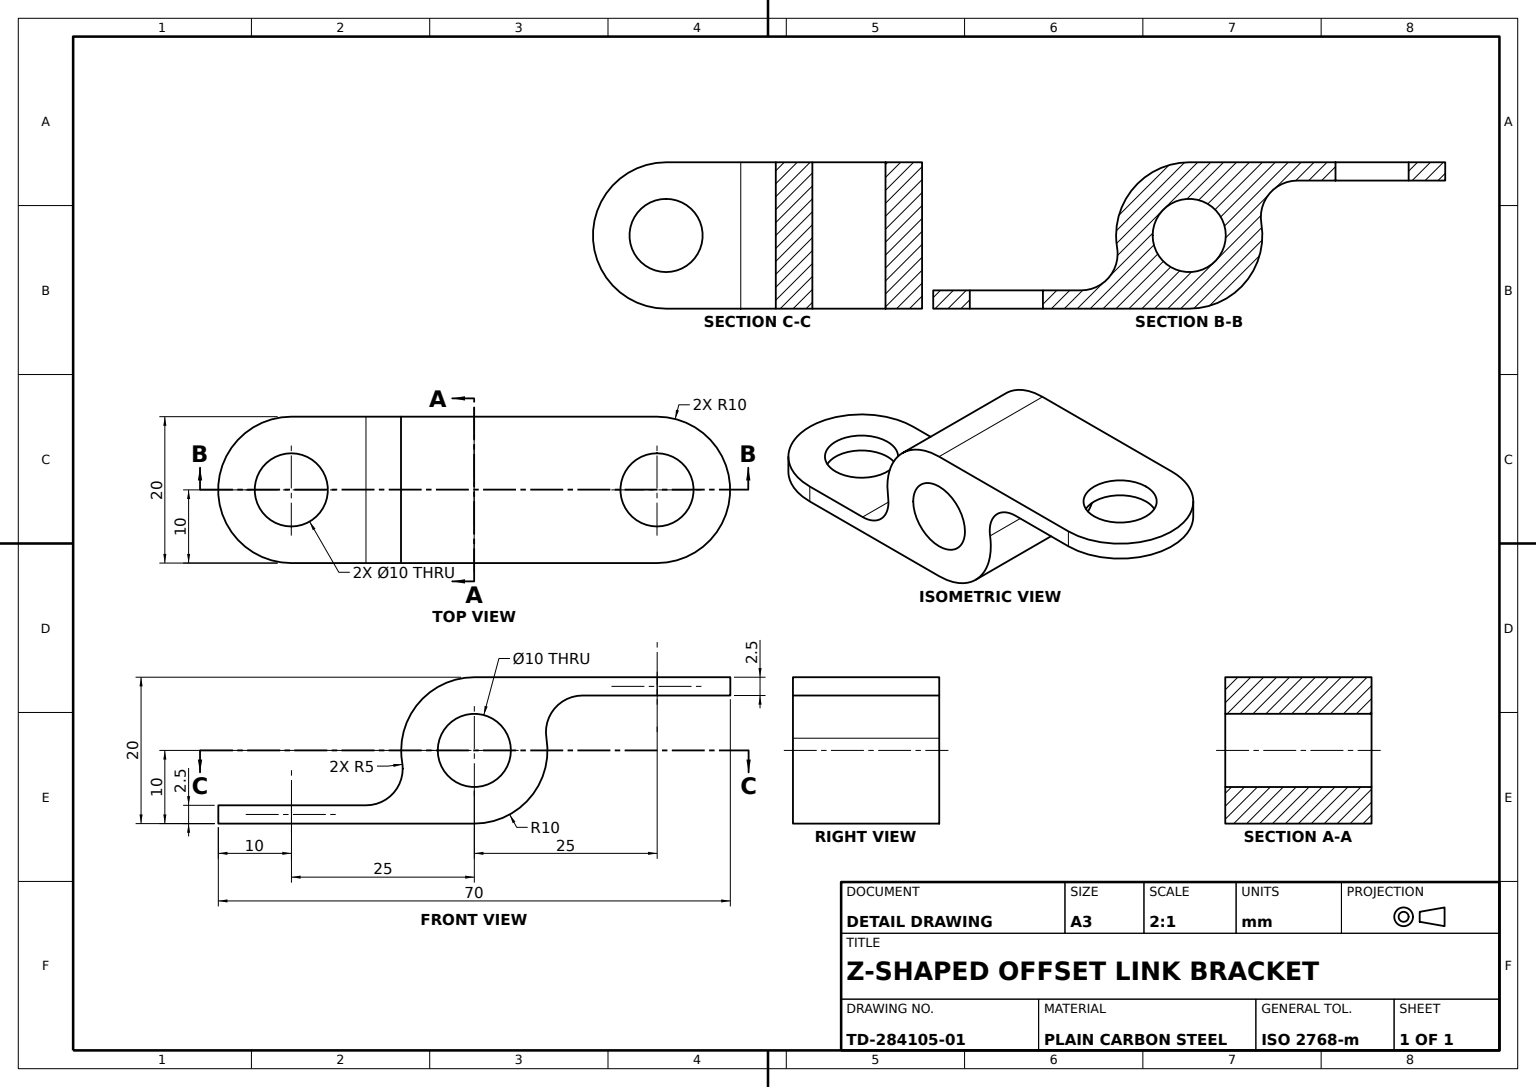
SolidWorks part; units mm, degrees
material "Plain Carbon Steel"
ref_plane "Front Plane" through (0, 0, 0) normal (0, 0, 1) x (1, 0, 0)
ref_plane "Top Plane" through (0, 0, 0) normal (0, 1, 0) x (1, 0, 0)
ref_plane "Right Plane" through (0, 0, 0) normal (1, 0, 0) x (0, 0, -1)
sketch "Hub Sketch Ø20" plane through (0, 0, 0) normal (0, 0, 1) x (1, 0, 0)
  circle A0 centre (0, 0) radius 10
  dimension "D1" = 20
  dimension "D2" = 20
extrude "Hub Cylinder Ø20" add sketch "Hub Sketch Ø20" along normal blind 20
sketch "First Arm Sketch" plane through (0, 0, 20) normal (0, 0, 1) x (1, 0, 0)
  line L0 (0, 10) -> (25, 10)
  line L1 (25, 10) -> (25, 7.5)
  line L2 (25, 7.5) -> (6.6144, 7.5)
  line L3 (0, -10) -> (-25, -10)
  line L4 (-25, -10) -> (-25, -7.5)
  line L5 (-25, -7.5) -> (-6.6144, -7.5)
  circle A0 centre (0, 0) radius 10 construction
  arc A1 (-6.6144, -7.5) -> (0, -10) centre (0, 0) ccw
  arc A2 (6.6144, 7.5) -> (0, 10) centre (0, 0) ccw
  dimension "D1" = 20
  dimension "D2" = 25
  dimension "D3" = 2.5
  dimension "D4" = 18.3856
  dimension "D5" = 18.3856
  dimension "D6" = 2.5
extrude "First Arm" add sketch "First Arm Sketch" against normal blind 20
sketch "Second Arm Sketch" plane through (0, 0, 20) normal (0, 0, 1) x (1, 0, 0)
  line L0 (14.7902, 7.5) -> (6.6144, 7.5)
  line L1 (-14.7902, -7.5) -> (-6.6144, -7.5)
  arc A1 (14.7902, 7.5) -> (9.8601, 1.6667) centre (14.7902, 2.5) ccw
  arc A2 (9.8601, 1.6667) -> (6.6144, 7.5) centre (0, 0) ccw
  arc A3 (-14.7902, -7.5) -> (-9.8601, -1.6667) centre (-14.7902, -2.5) ccw
  arc A4 (-9.8601, -1.6667) -> (-6.6144, -7.5) centre (0, 0) ccw
  arc A5 (9.8601, 1.6667) -> (6.6144, 7.5) centre (0, 0) ccw
  arc M4 (0, 10) -> (-6.6144, -7.5) centre (0, 0) ccw
  line M5 (-6.6144, -7.5) -> (-25, -7.5)
  arc M8 (0, -10) -> (6.6144, 7.5) centre (0, 0) ccw
  line M9 (6.6144, 7.5) -> (25, 7.5)
  dimension "D1" = 5
  dimension "D2" = 5
  dimension "D3" = 20
  dimension "D4" = 20
extrude "Second Arm" add sketch "Second Arm Sketch" against normal blind 20 contours A3 M5 M4 | A1 M9 M8
sketch "Tab A Sketch" plane through (0, -10, 0) normal (0, -1, 0) x (1, 0, 0)
  line L0 (-25, 0) -> (-25, 20) construction
  line L1 (-25, 20) -> (-25, 0)
  arc A0 (-25, 20) -> (-25, 0) centre (-25, 10) ccw
  dimension "D1" = 20
  dimension "D2" = 10
extrude "Tab A" add sketch "Tab A Sketch" against normal blind 2.5
sketch "Tab B Sketch" plane through (0, 10, 0) normal (0, 1, 0) x (1, 0, 0)
  line L0 (25, 0) -> (25, -20) construction
  line L1 (25, 0) -> (25, -20)
  arc A0 (25, -20) -> (25, 0) centre (25, -10) ccw
  dimension "D1" = 20
  dimension "D2" = 10
extrude "Tab B" add sketch "Tab B Sketch" against normal blind 2.5
sketch "Tab B Hole Sketch Ø10" plane through (0, 10, 0) normal (0, 1, 0) x (1, 0, 0)
  circle A0 centre (25, -10) radius 5
  dimension "D1" = 10
  dimension "D2" = 10
extrude "Tab B Hole Ø10" cut sketch "Tab B Hole Sketch Ø10" against normal blind 2.5
sketch "Tab A Hole Sketch Ø10" plane through (0, -10, 0) normal (0, -1, 0) x (1, 0, 0)
  circle A0 centre (-25, 10) radius 5
  dimension "D1" = 10
  dimension "D2" = 10
extrude "Tab A Hole Ø10" cut sketch "Tab A Hole Sketch Ø10" against normal blind 2.5
sketch "Hub Cross Bore Sketch Ø10" plane through (0, 0, 20) normal (0, 0, 1) x (1, 0, 0)
  circle A0 centre (0, 0) radius 5
  dimension "D1" = 10
  dimension "D2" = 10
extrude "Hub Cross Bore Ø10" cut sketch "Hub Cross Bore Sketch Ø10" against normal blind 20
